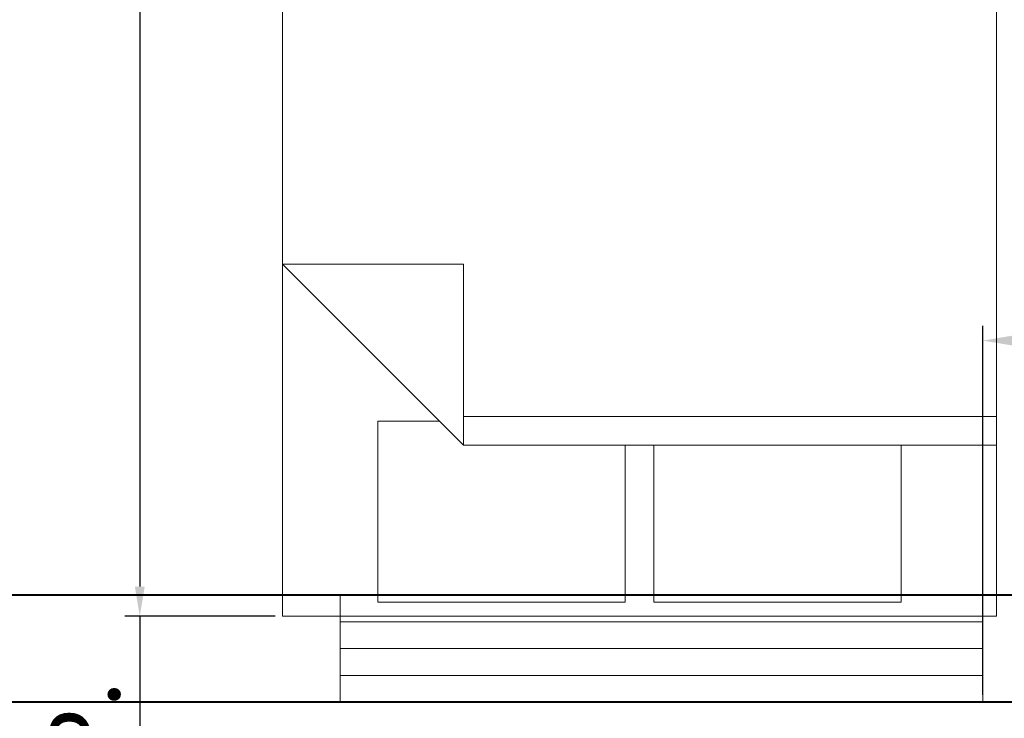
# Model space of a CAD drawing. Units: inches. Extents: x 459864 to 460310, y 324185 to 324787.
# Tile 70 of 112: x 460127 to 460210, y 324282 to 324341. Entities that reach past the tile are written whole.
import ezdxf

# ---------------------------------------------------------------- set-up
doc = ezdxf.new("R2010")
doc.units = ezdxf.units.IN
for name, color, linetype, lineweight in [('A-ANNO-DIMS', 2, 'Continuous', 18), ('A-FURN', 8, 'Continuous', 18), ('A-GLAZ', 4, 'Continuous', 18), ('A-WALL', 7, 'Continuous', 40), ('L-SITE-PATT', 252, 'Continuous', 13)]:
    doc.layers.add(name, color=color, linetype=linetype, lineweight=lineweight)
doc.styles.get("Standard").update_dxf_attribs({"font": 'arial.ttf'})
doc.dimstyles.new('ISO-25', dxfattribs={"dimtxt": 6, "dimasz": 2.5, "dimexe": 1.25, "dimexo": 0.625, "dimtad": 1, "dimdec": 1, "dimlunit": 3, "dimtxsty": 'Standard', "dimcen": 2.5, "dimadec": 0, "dimazin": 0, "dimtfac": 1, "dimtdec": 1, "dimtmove": 0, "dimatfit": 3, "dimfxl": 1, "dimarcsym": 0})

# ---------------------------------------------------------------- blocks, each defined once
blk = doc.blocks.new('Window - Wood Frame 36 in. Wide plan')
for p, q in [((0, 6), (0, 0)), ((36, 6), (36, 0)), ((0, 4.5), (36, 4.5)), ((0, 3), (36, 3)), ((0, 1.5), (36, 1.5))]:
    blk.add_line(p, q)
blk = doc.blocks.new('Bed - Queen')
for p, q in [((0, -80.00003), (0, 0)), ((0, 0), (59.99999, 0)), ((59.99999, 0), (59.99999, -80.00003)), ((7.99999, -1.2), (28.79998, -1.2)), ((7.99999, -14.4), (7.99999, -1.2)), ((28.79998, -1.2), (28.79998, -14.4)), ((31.19999, -1.2), (51.99999, -1.2)), ((31.19999, -14.4), (31.19999, -1.2)), ((51.99999, -1.2), (51.99999, -16.4)), ((0, -14.4), (44.8, -14.4)), ((59.99999, -29.6), (44.8, -14.4)), ((44.8, -14.4), (44.8, -29.6)), ((51.99999, -16.4), (46.79936, -16.4)), ((44.8, -16.8), (0, -16.8)), ((44.8, -29.6), (59.99999, -29.6)), ((59.99999, -80.00003), (0, -80.00003))]:
    blk.add_line(p, q)
blk = doc.blocks.new('*D28')
at = {"layer": 'A-ANNO-DIMS', "color": 0, "lineweight": -2, "transparency": 16777216}
for p, q in [((460148.65, 324370.7), (460136.025, 324370.7)), ((460137.275, 324368.2), (460137.275, 324293.2)), ((460148.65, 324290.7), (460136.025, 324290.7)), ((460137.275, 324290.7), (460137.275, 324198.69))]:
    blk.add_line(p, q, dxfattribs=at)
at = {"layer": 'A-ANNO-DIMS', "color": 0, "transparency": 16777216}
for points in [[(460136.858, 324368.2), (460137.692, 324368.2), (460137.275, 324370.7)], [(460136.858, 324293.2), (460137.692, 324293.2), (460137.275, 324290.7)]]:
    blk.add_solid(points, dxfattribs=at)
at = {"layer": 'Defpoints', "color": 0, "transparency": 16777216}
for p in [(460149.275, 324370.7), (460137.275, 324290.7), (460149.275, 324290.7)]:
    blk.add_point(p, dxfattribs=at)
at = {"layer": 'A-ANNO-DIMS', "color": 0, "transparency": 16777216, "insert": (460133.363, 324243.445), "char_height": 6, "attachment_point": 5, "rotation": 90}
blk.add_mtext('QUEEN BED 6\'-8" TYP.', dxfattribs=at)
blk = doc.blocks.new('*D67')
at = {"layer": 'A-ANNO-DIMS', "color": 0, "lineweight": -2, "transparency": 16777216}
for p, q in [((460208.115, 324284.108), (460208.115, 324315.133)), ((460247.115, 324284.108), (460247.115, 324315.133)), ((460210.615, 324313.883), (460244.615, 324313.883))]:
    blk.add_line(p, q, dxfattribs=at)
at = {"layer": 'A-ANNO-DIMS', "color": 0, "transparency": 16777216}
for points in [[(460210.615, 324314.3), (460210.615, 324313.467), (460208.115, 324313.883)], [(460244.615, 324314.3), (460244.615, 324313.467), (460247.115, 324313.883)]]:
    blk.add_solid(points, dxfattribs=at)
at = {"layer": 'Defpoints', "color": 0, "transparency": 16777216}
for p in [(460247.115, 324313.883), (460208.115, 324283.483), (460247.115, 324283.483)]:
    blk.add_point(p, dxfattribs=at)
at = {"layer": 'A-ANNO-DIMS', "color": 0, "transparency": 16777216, "insert": (460227.615, 324317.574), "char_height": 6, "attachment_point": 5}
blk.add_mtext('3\'-3"', dxfattribs=at)

msp = doc.modelspace()

# ---------------------------------------------------------------- hatches: boundary and pattern name
at = {"layer": 'L-SITE-PATT'}
h = msp.add_hatch(dxfattribs=at)
h.set_pattern_fill('DOTS', color=256)
h.paths.add_polyline_path([(460269.804, 324283.483), (460247.115, 324283.483), (460121.929, 324283.483), (460121.929, 324252.473), (460117.429, 324252.473), (460110.124, 324252.473), (460110.124, 324243.287), (460080.83, 324243.287), (460080.83, 324252.473), (460061.115, 324252.473), (460061.115, 324251.882), (460077.909, 324251.882), (460077.909, 324199.483), (460080.83, 324199.483), (460080.83, 324207.553), (460110.124, 324207.553), (460110.124, 324199.483), (460110.813, 324199.483), (460262.115, 324199.483), (460269.804, 324199.483)], flags=17)
edge = h.paths.add_edge_path(flags=0)
edge.add_ellipse((460222.59, 324263.813), major_axis=(-8.485, 8.485), ratio=1, start_angle=405, end_angle=495, ccw=False)
edge.add_line((460214.821, 324254.66), (460214.832, 324254.666))
edge.add_ellipse((460222.59, 324263.813), major_axis=(-8.485, 8.485), ratio=1, start_angle=405, end_angle=495, ccw=False)
edge.add_line((460210.759, 324261.781), (460210.768, 324261.787))
edge.add_ellipse((460222.59, 324263.813), major_axis=(-8.485, 8.485), ratio=1, start_angle=405, end_angle=495, ccw=False)
edge.add_ellipse((460222.59, 324263.813), major_axis=(-8.485, 8.485), ratio=1, start_angle=392.75402, end_angle=405, ccw=False)
edge.add_ellipse((460222.59, 324263.813), major_axis=(-8.485, 8.485), ratio=1, start_angle=380.93472, end_angle=392.75402, ccw=False)
edge.add_line((460211.337, 324267.985), (460211.34, 324267.985))
edge.add_ellipse((460222.59, 324263.813), major_axis=(-8.485, 8.485), ratio=1, start_angle=380.93472, end_angle=392.75402, ccw=False)
edge.add_ellipse((460222.59, 324263.813), major_axis=(-8.485, 8.485), ratio=1, start_angle=347.90152, end_angle=380.93472, ccw=False)
edge.add_ellipse((460222.59, 324263.813), major_axis=(-8.485, 8.485), ratio=1, start_angle=327.06192, end_angle=347.90152, ccw=False)
edge.add_ellipse((460222.59, 324263.813), major_axis=(-8.485, 8.485), ratio=1, start_angle=278.32464, end_angle=327.06192, ccw=False)
edge.add_line((460225.158, 324275.536), (460225.158, 324275.535))
edge.add_ellipse((460222.59, 324263.813), major_axis=(-8.485, 8.485), ratio=1, start_angle=278.32464, end_angle=327.06192, ccw=False)
edge.add_ellipse((460222.59, 324263.813), major_axis=(-8.485, 8.485), ratio=1, start_angle=260.64357, end_angle=278.32464, ccw=False)
edge.add_ellipse((460222.59, 324263.813), major_axis=(-8.485, 8.485), ratio=1, start_angle=225, end_angle=260.64357, ccw=False)
edge.add_line((460234.509, 324265.243), (460234.501, 324265.239))
edge.add_ellipse((460222.59, 324263.813), major_axis=(-8.485, 8.485), ratio=1, start_angle=225, end_angle=260.64357, ccw=False)
edge.add_ellipse((460222.59, 324263.813), major_axis=(-8.485, 8.485), ratio=1, start_angle=495, end_angle=585, ccw=False)
edge.add_line((460234.437, 324261.861), (460234.424, 324261.858))
edge.add_ellipse((460222.59, 324263.813), major_axis=(-8.485, 8.485), ratio=1, start_angle=495, end_angle=585, ccw=False)
edge.add_line((460227.95, 324253.067), (460227.946, 324253.083))
edge.add_ellipse((460222.59, 324263.813), major_axis=(-8.485, 8.485), ratio=1, start_angle=495, end_angle=585, ccw=False)
edge.add_line((460226.223, 324252.369), (460226.211, 324252.38))
edge.add_ellipse((460222.59, 324263.813), major_axis=(-8.485, 8.485), ratio=1, start_angle=495, end_angle=585, ccw=False)
h.paths.add_polyline_path([(460219.651, 324254.347), (460218.461, 324253.545), (460218.275, 324254.789), (460219.642, 324256.542), (460219.625, 324260.848), (460216.11, 324257.333), (460214.35, 324256.978), (460215.416, 324259.356), (460212.524, 324258.496), (460213.137, 324259.93), (460218.507, 324263.813), (460222.59, 324263.813), (460222.59, 324267.807), (460218.176, 324272.212), (460219.026, 324274.639), (460222.59, 324272.811), (460222.59, 324275.423), (460223.057, 324274.825), (460222.675, 324273.492), (460225.912, 324267.135), (460219.625, 324260.848)], flags=0)
edge = h.paths.add_edge_path(flags=0)
edge.add_ellipse((460194.576, 324264.046), major_axis=(-8.485, 8.485), ratio=1, start_angle=495, end_angle=585, ccw=False)
edge.add_line((460199.936, 324253.3), (460199.932, 324253.316))
edge.add_ellipse((460194.576, 324264.046), major_axis=(-8.485, 8.485), ratio=1, start_angle=495, end_angle=585, ccw=False)
edge.add_line((460198.208, 324252.603), (460198.196, 324252.613))
edge.add_ellipse((460194.576, 324264.046), major_axis=(-8.485, 8.485), ratio=1, start_angle=495, end_angle=585, ccw=False)
edge.add_ellipse((460194.576, 324264.046), major_axis=(-8.485, 8.485), ratio=1, start_angle=405, end_angle=495, ccw=False)
edge.add_line((460186.806, 324254.893), (460186.817, 324254.899))
edge.add_ellipse((460194.576, 324264.046), major_axis=(-8.485, 8.485), ratio=1, start_angle=405, end_angle=495, ccw=False)
edge.add_line((460182.744, 324262.014), (460182.753, 324262.02))
edge.add_ellipse((460194.576, 324264.046), major_axis=(-8.485, 8.485), ratio=1, start_angle=405, end_angle=495, ccw=False)
edge.add_ellipse((460194.576, 324264.046), major_axis=(-8.485, 8.485), ratio=1, start_angle=392.75402, end_angle=405, ccw=False)
edge.add_ellipse((460194.576, 324264.046), major_axis=(-8.485, 8.485), ratio=1, start_angle=380.93472, end_angle=392.75402, ccw=False)
edge.add_line((460183.323, 324268.218), (460183.326, 324268.218))
edge.add_ellipse((460194.576, 324264.046), major_axis=(-8.485, 8.485), ratio=1, start_angle=380.93472, end_angle=392.75402, ccw=False)
edge.add_ellipse((460194.576, 324264.046), major_axis=(-8.485, 8.485), ratio=1, start_angle=347.90152, end_angle=380.93472, ccw=False)
edge.add_ellipse((460194.576, 324264.046), major_axis=(-8.485, 8.485), ratio=1, start_angle=327.06192, end_angle=347.90152, ccw=False)
edge.add_ellipse((460194.576, 324264.046), major_axis=(-8.485, 8.485), ratio=1, start_angle=278.32464, end_angle=327.06192, ccw=False)
edge.add_line((460197.144, 324275.769), (460197.143, 324275.768))
edge.add_ellipse((460194.576, 324264.046), major_axis=(-8.485, 8.485), ratio=1, start_angle=278.32464, end_angle=327.06192, ccw=False)
edge.add_ellipse((460194.576, 324264.046), major_axis=(-8.485, 8.485), ratio=1, start_angle=260.64357, end_angle=278.32464, ccw=False)
edge.add_ellipse((460194.576, 324264.046), major_axis=(-8.485, 8.485), ratio=1, start_angle=225, end_angle=260.64357, ccw=False)
edge.add_line((460206.494, 324265.476), (460206.487, 324265.473))
edge.add_ellipse((460194.576, 324264.046), major_axis=(-8.485, 8.485), ratio=1, start_angle=225, end_angle=260.64357, ccw=False)
edge.add_ellipse((460194.576, 324264.046), major_axis=(-8.485, 8.485), ratio=1, start_angle=495, end_angle=585, ccw=False)
edge.add_line((460206.422, 324262.094), (460206.409, 324262.091))
h.paths.add_polyline_path([(460191.61, 324261.081), (460191.637, 324254.58), (460190.447, 324253.778), (460190.261, 324255.023), (460191.628, 324256.775), (460191.61, 324261.081), (460188.096, 324257.566), (460186.335, 324257.211), (460187.402, 324259.589), (460184.509, 324258.729), (460185.123, 324260.163), (460190.493, 324264.046), (460194.576, 324264.046), (460194.576, 324268.04), (460190.161, 324272.446), (460191.011, 324274.872), (460194.576, 324273.044), (460194.576, 324275.657), (460195.043, 324275.058), (460194.661, 324273.725), (460197.897, 324267.368)], flags=0)
edge = h.paths.add_edge_path(flags=0)
edge.add_ellipse((460252.912, 324263.578), major_axis=(-8.485, 8.485), ratio=1, start_angle=405, end_angle=495, ccw=False)
edge.add_line((460241.081, 324261.545), (460241.089, 324261.551))
edge.add_ellipse((460252.912, 324263.578), major_axis=(-8.485, 8.485), ratio=1, start_angle=405, end_angle=495, ccw=False)
edge.add_ellipse((460252.912, 324263.578), major_axis=(-8.485, 8.485), ratio=1, start_angle=392.75402, end_angle=405, ccw=False)
edge.add_ellipse((460252.912, 324263.578), major_axis=(-8.485, 8.485), ratio=1, start_angle=380.93472, end_angle=392.75402, ccw=False)
edge.add_line((460241.659, 324267.749), (460241.662, 324267.749))
edge.add_ellipse((460252.912, 324263.578), major_axis=(-8.485, 8.485), ratio=1, start_angle=380.93472, end_angle=392.75402, ccw=False)
edge.add_ellipse((460252.912, 324263.578), major_axis=(-8.485, 8.485), ratio=1, start_angle=347.90152, end_angle=380.93472, ccw=False)
edge.add_ellipse((460252.912, 324263.578), major_axis=(-8.485, 8.485), ratio=1, start_angle=327.06192, end_angle=347.90152, ccw=False)
edge.add_ellipse((460252.912, 324263.578), major_axis=(-8.485, 8.485), ratio=1, start_angle=278.32464, end_angle=327.06192, ccw=False)
edge.add_line((460255.48, 324275.3), (460255.479, 324275.299))
edge.add_ellipse((460252.912, 324263.578), major_axis=(-8.485, 8.485), ratio=1, start_angle=278.32464, end_angle=327.06192, ccw=False)
edge.add_ellipse((460252.912, 324263.578), major_axis=(-8.485, 8.485), ratio=1, start_angle=260.64357, end_angle=278.32464, ccw=False)
edge.add_ellipse((460252.912, 324263.578), major_axis=(-8.485, 8.485), ratio=1, start_angle=225, end_angle=260.64357, ccw=False)
edge.add_line((460264.83, 324265.007), (460264.823, 324265.004))
edge.add_ellipse((460252.912, 324263.578), major_axis=(-8.485, 8.485), ratio=1, start_angle=225, end_angle=260.64357, ccw=False)
edge.add_ellipse((460252.912, 324263.578), major_axis=(-8.485, 8.485), ratio=1, start_angle=495, end_angle=585, ccw=False)
edge.add_line((460264.758, 324261.626), (460264.745, 324261.622))
edge.add_ellipse((460252.912, 324263.578), major_axis=(-8.485, 8.485), ratio=1, start_angle=495, end_angle=585, ccw=False)
edge.add_line((460258.272, 324252.832), (460258.268, 324252.848))
edge.add_ellipse((460252.912, 324263.578), major_axis=(-8.485, 8.485), ratio=1, start_angle=495, end_angle=585, ccw=False)
edge.add_line((460256.545, 324252.134), (460256.533, 324252.144))
edge.add_ellipse((460252.912, 324263.578), major_axis=(-8.485, 8.485), ratio=1, start_angle=495, end_angle=585, ccw=False)
edge.add_ellipse((460252.912, 324263.578), major_axis=(-8.485, 8.485), ratio=1, start_angle=405, end_angle=495, ccw=False)
edge.add_line((460245.143, 324254.424), (460245.153, 324254.43))
h.paths.add_polyline_path([(460244.672, 324256.742), (460245.738, 324259.12), (460242.846, 324258.26), (460243.459, 324259.694), (460248.829, 324263.578), (460252.912, 324263.578), (460252.912, 324267.571), (460248.497, 324271.977), (460249.348, 324274.403), (460252.912, 324272.576), (460252.912, 324275.188), (460253.379, 324274.589), (460252.997, 324273.257), (460256.233, 324266.899), (460249.946, 324260.612), (460249.973, 324254.111), (460248.783, 324253.309), (460248.597, 324254.554), (460249.964, 324256.306), (460249.946, 324260.612), (460246.432, 324257.097)], flags=0)
edge = h.paths.add_edge_path(flags=0)
edge.add_ellipse((460167.439, 324262.833), major_axis=(-8.485, 8.485), ratio=1, start_angle=495, end_angle=585, ccw=False)
edge.add_line((460172.799, 324252.087), (460172.795, 324252.103))
edge.add_ellipse((460167.439, 324262.833), major_axis=(-8.485, 8.485), ratio=1, start_angle=495, end_angle=585, ccw=False)
edge.add_line((460171.071, 324251.389), (460171.059, 324251.399))
edge.add_ellipse((460167.439, 324262.833), major_axis=(-8.485, 8.485), ratio=1, start_angle=495, end_angle=585, ccw=False)
edge.add_ellipse((460167.439, 324262.833), major_axis=(-8.485, 8.485), ratio=1, start_angle=405, end_angle=495, ccw=False)
edge.add_line((460159.669, 324253.679), (460159.68, 324253.685))
edge.add_ellipse((460167.439, 324262.833), major_axis=(-8.485, 8.485), ratio=1, start_angle=405, end_angle=495, ccw=False)
edge.add_line((460155.607, 324260.8), (460155.616, 324260.806))
edge.add_ellipse((460167.439, 324262.833), major_axis=(-8.485, 8.485), ratio=1, start_angle=405, end_angle=495, ccw=False)
edge.add_ellipse((460167.439, 324262.833), major_axis=(-8.485, 8.485), ratio=1, start_angle=392.75402, end_angle=405, ccw=False)
edge.add_ellipse((460167.439, 324262.833), major_axis=(-8.485, 8.485), ratio=1, start_angle=380.93472, end_angle=392.75402, ccw=False)
edge.add_line((460156.185, 324267.005), (460156.189, 324267.005))
edge.add_ellipse((460167.439, 324262.833), major_axis=(-8.485, 8.485), ratio=1, start_angle=380.93472, end_angle=392.75402, ccw=False)
edge.add_ellipse((460167.439, 324262.833), major_axis=(-8.485, 8.485), ratio=1, start_angle=347.90152, end_angle=380.93472, ccw=False)
edge.add_ellipse((460167.439, 324262.833), major_axis=(-8.485, 8.485), ratio=1, start_angle=327.06192, end_angle=347.90152, ccw=False)
edge.add_ellipse((460167.439, 324262.833), major_axis=(-8.485, 8.485), ratio=1, start_angle=278.32464, end_angle=327.06192, ccw=False)
edge.add_line((460170.007, 324274.556), (460170.006, 324274.554))
edge.add_ellipse((460167.439, 324262.833), major_axis=(-8.485, 8.485), ratio=1, start_angle=278.32464, end_angle=327.06192, ccw=False)
edge.add_ellipse((460167.439, 324262.833), major_axis=(-8.485, 8.485), ratio=1, start_angle=260.64357, end_angle=278.32464, ccw=False)
edge.add_ellipse((460167.439, 324262.833), major_axis=(-8.485, 8.485), ratio=1, start_angle=225, end_angle=260.64357, ccw=False)
edge.add_line((460179.357, 324264.262), (460179.35, 324264.259))
edge.add_ellipse((460167.439, 324262.833), major_axis=(-8.485, 8.485), ratio=1, start_angle=225, end_angle=260.64357, ccw=False)
edge.add_ellipse((460167.439, 324262.833), major_axis=(-8.485, 8.485), ratio=1, start_angle=495, end_angle=585, ccw=False)
edge.add_line((460179.285, 324260.881), (460179.272, 324260.877))
h.paths.add_polyline_path([(460164.473, 324259.867), (460164.5, 324253.366), (460163.31, 324252.565), (460163.124, 324253.809), (460164.491, 324255.561), (460164.473, 324259.867), (460160.958, 324256.353), (460159.198, 324255.998), (460160.265, 324258.375), (460157.372, 324257.515), (460157.986, 324258.949), (460163.356, 324262.833), (460167.439, 324262.833), (460167.439, 324266.826), (460163.024, 324271.232), (460163.874, 324273.659), (460167.439, 324271.831), (460167.439, 324274.443), (460167.905, 324273.844), (460167.524, 324272.512), (460170.76, 324266.154)], flags=0)
edge = h.paths.add_edge_path(flags=0)
edge.add_ellipse((460140.758, 324262.37), major_axis=(-8.485, 8.485), ratio=1, start_angle=495, end_angle=585, ccw=False)
edge.add_line((460146.118, 324251.624), (460146.114, 324251.639))
edge.add_ellipse((460140.758, 324262.37), major_axis=(-8.485, 8.485), ratio=1, start_angle=495, end_angle=585, ccw=False)
edge.add_line((460144.391, 324250.926), (460144.379, 324250.936))
edge.add_ellipse((460140.758, 324262.37), major_axis=(-8.485, 8.485), ratio=1, start_angle=495, end_angle=585, ccw=False)
edge.add_ellipse((460140.758, 324262.37), major_axis=(-8.485, 8.485), ratio=1, start_angle=405, end_angle=495, ccw=False)
edge.add_line((460132.989, 324253.216), (460132.999, 324253.222))
edge.add_ellipse((460140.758, 324262.37), major_axis=(-8.485, 8.485), ratio=1, start_angle=405, end_angle=495, ccw=False)
edge.add_line((460128.927, 324260.337), (460128.935, 324260.343))
edge.add_ellipse((460140.758, 324262.37), major_axis=(-8.485, 8.485), ratio=1, start_angle=405, end_angle=495, ccw=False)
edge.add_ellipse((460140.758, 324262.37), major_axis=(-8.485, 8.485), ratio=1, start_angle=392.75402, end_angle=405, ccw=False)
edge.add_ellipse((460140.758, 324262.37), major_axis=(-8.485, 8.485), ratio=1, start_angle=380.93472, end_angle=392.75402, ccw=False)
edge.add_line((460129.505, 324266.541), (460129.508, 324266.541))
edge.add_ellipse((460140.758, 324262.37), major_axis=(-8.485, 8.485), ratio=1, start_angle=380.93472, end_angle=392.75402, ccw=False)
edge.add_ellipse((460140.758, 324262.37), major_axis=(-8.485, 8.485), ratio=1, start_angle=347.90152, end_angle=380.93472, ccw=False)
edge.add_ellipse((460140.758, 324262.37), major_axis=(-8.485, 8.485), ratio=1, start_angle=327.06192, end_angle=347.90152, ccw=False)
edge.add_ellipse((460140.758, 324262.37), major_axis=(-8.485, 8.485), ratio=1, start_angle=278.32464, end_angle=327.06192, ccw=False)
edge.add_line((460143.326, 324274.092), (460143.325, 324274.091))
edge.add_ellipse((460140.758, 324262.37), major_axis=(-8.485, 8.485), ratio=1, start_angle=278.32464, end_angle=327.06192, ccw=False)
edge.add_ellipse((460140.758, 324262.37), major_axis=(-8.485, 8.485), ratio=1, start_angle=260.64357, end_angle=278.32464, ccw=False)
edge.add_ellipse((460140.758, 324262.37), major_axis=(-8.485, 8.485), ratio=1, start_angle=225, end_angle=260.64357, ccw=False)
edge.add_line((460152.677, 324263.799), (460152.669, 324263.796))
edge.add_ellipse((460140.758, 324262.37), major_axis=(-8.485, 8.485), ratio=1, start_angle=225, end_angle=260.64357, ccw=False)
edge.add_ellipse((460140.758, 324262.37), major_axis=(-8.485, 8.485), ratio=1, start_angle=495, end_angle=585, ccw=False)
edge.add_line((460152.604, 324260.418), (460152.592, 324260.414))
h.paths.add_polyline_path([(460137.792, 324259.404), (460137.819, 324252.903), (460136.629, 324252.101), (460136.443, 324253.346), (460137.81, 324255.098), (460137.792, 324259.404), (460134.278, 324255.889), (460132.518, 324255.534), (460133.584, 324257.912), (460130.692, 324257.052), (460131.305, 324258.486), (460136.675, 324262.37), (460140.758, 324262.37), (460140.758, 324266.363), (460136.343, 324270.769), (460137.194, 324273.195), (460140.758, 324271.367), (460140.758, 324273.98), (460141.225, 324273.381), (460140.843, 324272.049), (460144.079, 324265.691)], flags=0)
h.paths.add_polyline_path([(460110.124, 324227.414), (460080.83, 324227.414), (460080.83, 324235.484), (460110.124, 324235.484)], flags=16)
h.paths.add_polyline_path([(460110.124, 324220.797), (460110.124, 324212.727), (460080.83, 324212.727), (460080.83, 324220.797)], flags=16)
h.paths.add_polyline_path([(460269.804, 324283.483), (460247.115, 324283.483), (460121.929, 324283.483), (460121.929, 324252.473), (460117.429, 324252.473), (460110.124, 324252.473), (460110.124, 324243.287), (460080.83, 324243.287), (460080.83, 324252.473), (460061.115, 324252.473), (460061.115, 324251.882), (460077.909, 324251.882), (460077.909, 324199.483), (460080.83, 324199.483), (460080.83, 324207.553), (460110.124, 324207.553), (460110.124, 324199.483), (460262.115, 324199.483), (460269.804, 324199.483)], flags=17)
h.paths.add_polyline_path([(460219.651, 324254.347), (460218.461, 324253.545), (460218.275, 324254.789), (460219.642, 324256.542), (460219.625, 324260.848), (460216.11, 324257.333), (460214.35, 324256.978), (460215.416, 324259.356), (460212.524, 324258.496), (460213.137, 324259.93), (460218.507, 324263.813), (460222.59, 324263.813), (460220.18, 324266.223), (460215.461, 324265.308), (460211.835, 324266.137), (460216.247, 324267.985), (460218.418, 324267.985), (460222.59, 324263.813), (460222.59, 324267.807), (460218.176, 324272.212), (460219.026, 324274.639), (460222.59, 324272.811), (460222.59, 324275.423), (460223.057, 324274.825), (460222.675, 324273.492), (460225.912, 324267.135), (460222.59, 324263.813), (460231.383, 324263.813), (460228.485, 324262.488), (460224.425, 324261.978), (460228.68, 324257.724), (460228.966, 324254.791), (460227.142, 324256.537), (460227.542, 324254.819), (460227.333, 324253.614), (460222.59, 324259.985), (460222.59, 324255.497), (460221.377, 324256.541), (460220.576, 324261.799), (460219.625, 324260.848)], flags=0)
h.paths.add_polyline_path([(460199.127, 324256.77), (460199.528, 324255.052), (460199.319, 324253.848), (460194.576, 324260.218), (460194.576, 324255.73), (460193.363, 324256.774), (460192.561, 324262.032), (460191.61, 324261.081), (460191.637, 324254.58), (460190.447, 324253.778), (460190.261, 324255.023), (460191.628, 324256.775), (460191.61, 324261.081), (460188.096, 324257.566), (460186.335, 324257.211), (460187.402, 324259.589), (460184.509, 324258.729), (460185.123, 324260.163), (460190.493, 324264.046), (460194.576, 324264.046), (460192.166, 324266.456), (460187.446, 324265.541), (460183.82, 324266.37), (460188.232, 324268.218), (460190.404, 324268.218), (460194.576, 324264.046), (460194.576, 324268.04), (460190.161, 324272.446), (460191.011, 324274.872), (460194.576, 324273.044), (460194.576, 324275.657), (460195.043, 324275.058), (460194.661, 324273.725), (460197.897, 324267.368), (460194.576, 324264.046), (460203.368, 324264.046), (460200.47, 324262.721), (460196.411, 324262.212), (460200.665, 324257.957), (460200.951, 324255.024)], flags=0)
h.paths.add_polyline_path([(460244.672, 324256.742), (460245.738, 324259.12), (460242.846, 324258.26), (460243.459, 324259.694), (460248.829, 324263.578), (460252.912, 324263.578), (460250.502, 324265.987), (460245.783, 324265.072), (460242.156, 324265.901), (460246.568, 324267.749), (460248.74, 324267.749), (460252.912, 324263.578), (460252.912, 324267.571), (460248.497, 324271.977), (460249.348, 324274.403), (460252.912, 324272.576), (460252.912, 324275.188), (460253.379, 324274.589), (460252.997, 324273.257), (460256.233, 324266.899), (460252.912, 324263.578), (460261.705, 324263.578), (460258.806, 324262.252), (460254.747, 324261.743), (460259.002, 324257.488), (460259.288, 324254.555), (460257.463, 324256.301), (460257.864, 324254.583), (460257.655, 324253.379), (460252.912, 324259.749), (460252.912, 324255.261), (460251.699, 324256.305), (460250.897, 324261.563), (460249.946, 324260.612), (460249.973, 324254.111), (460248.783, 324253.309), (460248.597, 324254.554), (460249.964, 324256.306), (460249.946, 324260.612), (460246.432, 324257.097)], flags=0)
h.paths.add_polyline_path([(460173.528, 324256.743), (460173.814, 324253.811), (460171.99, 324255.556), (460172.39, 324253.838), (460172.182, 324252.634), (460167.439, 324259.004), (460167.439, 324254.516), (460166.226, 324255.56), (460165.424, 324260.818), (460164.473, 324259.867), (460164.5, 324253.366), (460163.31, 324252.565), (460163.124, 324253.809), (460164.491, 324255.561), (460164.473, 324259.867), (460160.958, 324256.353), (460159.198, 324255.998), (460160.265, 324258.375), (460157.372, 324257.515), (460157.986, 324258.949), (460163.356, 324262.833), (460167.439, 324262.833), (460165.029, 324265.243), (460160.309, 324264.327), (460156.683, 324265.156), (460161.095, 324267.005), (460163.267, 324267.005), (460167.439, 324262.833), (460167.439, 324266.826), (460163.024, 324271.232), (460163.874, 324273.659), (460167.439, 324271.831), (460167.439, 324274.443), (460167.905, 324273.844), (460167.524, 324272.512), (460170.76, 324266.154), (460167.439, 324262.833), (460176.231, 324262.833), (460173.333, 324261.507), (460169.274, 324260.998)], flags=0)
h.paths.add_polyline_path([(460146.848, 324256.28), (460147.134, 324253.347), (460145.31, 324255.093), (460145.71, 324253.375), (460145.501, 324252.171), (460140.758, 324258.541), (460140.758, 324254.053), (460139.545, 324255.097), (460138.744, 324260.355), (460137.792, 324259.404), (460137.819, 324252.903), (460136.629, 324252.101), (460136.443, 324253.346), (460137.81, 324255.098), (460137.792, 324259.404), (460134.278, 324255.889), (460132.518, 324255.534), (460133.584, 324257.912), (460130.692, 324257.052), (460131.305, 324258.486), (460136.675, 324262.37), (460140.758, 324262.37), (460138.348, 324264.779), (460133.629, 324263.864), (460130.002, 324264.693), (460134.414, 324266.541), (460136.586, 324266.541), (460140.758, 324262.37), (460140.758, 324266.363), (460136.343, 324270.769), (460137.194, 324273.195), (460140.758, 324271.367), (460140.758, 324273.98), (460141.225, 324273.381), (460140.843, 324272.049), (460144.079, 324265.691), (460140.758, 324262.37), (460149.551, 324262.37), (460146.653, 324261.044), (460142.593, 324260.535)], flags=0)
edge = h.paths.add_edge_path()
edge.add_line((460269.804, 324272.549), (460260.881, 324272.549))
edge.add_ellipse((460252.912, 324263.578), major_axis=(-8.485, 8.485), ratio=1, start_angle=260.64357, end_angle=273.38462, ccw=False)
edge.add_line((460262.283, 324271.092), (460262.261, 324271.091))
edge.add_ellipse((460252.912, 324263.578), major_axis=(-8.485, 8.485), ratio=1, start_angle=260.64357, end_angle=273.38462, ccw=False)
edge.add_ellipse((460252.912, 324263.578), major_axis=(-8.485, 8.485), ratio=1, start_angle=225, end_angle=260.64357, ccw=False)
edge.add_line((460263.609, 324269.063), (460263.572, 324269.058))
edge.add_ellipse((460252.912, 324263.578), major_axis=(-8.485, 8.485), ratio=1, start_angle=225, end_angle=260.64357, ccw=False)
edge.add_line((460264.615, 324266.306), (460264.585, 324266.305))
edge.add_ellipse((460252.912, 324263.578), major_axis=(-8.485, 8.485), ratio=1, start_angle=225, end_angle=260.64357, ccw=False)
edge.add_line((460264.83, 324265.007), (460264.823, 324265.004))
edge.add_ellipse((460252.912, 324263.578), major_axis=(-8.485, 8.485), ratio=1, start_angle=225, end_angle=260.64357, ccw=False)
edge.add_ellipse((460252.912, 324263.578), major_axis=(-8.485, 8.485), ratio=1, start_angle=495, end_angle=585, ccw=False)
edge.add_line((460264.758, 324261.626), (460264.745, 324261.622))
edge.add_ellipse((460252.912, 324263.578), major_axis=(-8.485, 8.485), ratio=1, start_angle=495, end_angle=585, ccw=False)
edge.add_line((460263.442, 324257.739), (460263.389, 324257.779))
edge.add_ellipse((460252.912, 324263.578), major_axis=(-8.485, 8.485), ratio=1, start_angle=495, end_angle=585, ccw=False)
edge.add_line((460258.128, 324252.744), (460258.102, 324252.779))
edge.add_ellipse((460252.912, 324263.578), major_axis=(-8.485, 8.485), ratio=1, start_angle=495, end_angle=585, ccw=False)
edge.add_line((460256.545, 324252.134), (460256.533, 324252.144))
edge.add_ellipse((460252.912, 324263.578), major_axis=(-8.485, 8.485), ratio=1, start_angle=495, end_angle=585, ccw=False)
edge.add_ellipse((460252.912, 324263.578), major_axis=(-8.485, 8.485), ratio=1, start_angle=405, end_angle=495, ccw=False)
edge.add_line((460250.594, 324251.78), (460250.605, 324251.82))
edge.add_ellipse((460252.912, 324263.578), major_axis=(-8.485, 8.485), ratio=1, start_angle=405, end_angle=495, ccw=False)
edge.add_line((460245.143, 324254.424), (460245.153, 324254.43))
edge.add_ellipse((460252.912, 324263.578), major_axis=(-8.485, 8.485), ratio=1, start_angle=405, end_angle=495, ccw=False)
edge.add_line((460243.525, 324256.059), (460243.56, 324256.091))
edge.add_ellipse((460252.912, 324263.578), major_axis=(-8.485, 8.485), ratio=1, start_angle=405, end_angle=495, ccw=False)
edge.add_line((460241.44, 324259.893), (460241.522, 324259.896))
edge.add_ellipse((460252.912, 324263.578), major_axis=(-8.485, 8.485), ratio=1, start_angle=405, end_angle=495, ccw=False)
edge.add_line((460241.081, 324261.545), (460241.089, 324261.551))
edge.add_ellipse((460252.912, 324263.578), major_axis=(-8.485, 8.485), ratio=1, start_angle=405, end_angle=495, ccw=False)
edge.add_ellipse((460252.912, 324263.578), major_axis=(-8.485, 8.485), ratio=1, start_angle=392.75402, end_angle=405, ccw=False)
edge.add_line((460241.05, 324265.438), (460241.063, 324265.443))
edge.add_ellipse((460252.912, 324263.578), major_axis=(-8.485, 8.485), ratio=1, start_angle=392.75402, end_angle=405, ccw=False)
edge.add_ellipse((460252.912, 324263.578), major_axis=(-8.485, 8.485), ratio=1, start_angle=380.93472, end_angle=392.75402, ccw=False)
edge.add_line((460241.452, 324267.176), (460241.469, 324267.171))
edge.add_ellipse((460252.912, 324263.578), major_axis=(-8.485, 8.485), ratio=1, start_angle=380.93472, end_angle=392.75402, ccw=False)
edge.add_line((460241.659, 324267.749), (460241.662, 324267.749))
edge.add_ellipse((460252.912, 324263.578), major_axis=(-8.485, 8.485), ratio=1, start_angle=380.93472, end_angle=392.75402, ccw=False)
edge.add_ellipse((460252.912, 324263.578), major_axis=(-8.485, 8.485), ratio=1, start_angle=356.61538, end_angle=380.93472, ccw=False)
edge.add_line((460244.88, 324272.488), (460244.713, 324272.549))
edge.add_line((460244.713, 324272.549), (460230.817, 324272.549))
edge.add_ellipse((460222.59, 324263.813), major_axis=(-8.485, 8.485), ratio=1, start_angle=260.64357, end_angle=271.71777, ccw=False)
edge.add_ellipse((460222.59, 324263.813), major_axis=(-8.485, 8.485), ratio=1, start_angle=225, end_angle=260.64357, ccw=False)
edge.add_line((460233.287, 324269.299), (460233.25, 324269.294))
edge.add_ellipse((460222.59, 324263.813), major_axis=(-8.485, 8.485), ratio=1, start_angle=225, end_angle=260.64357, ccw=False)
edge.add_line((460234.294, 324266.541), (460234.264, 324266.541))
edge.add_ellipse((460222.59, 324263.813), major_axis=(-8.485, 8.485), ratio=1, start_angle=225, end_angle=260.64357, ccw=False)
edge.add_line((460234.509, 324265.243), (460234.501, 324265.239))
edge.add_ellipse((460222.59, 324263.813), major_axis=(-8.485, 8.485), ratio=1, start_angle=225, end_angle=260.64357, ccw=False)
edge.add_ellipse((460222.59, 324263.813), major_axis=(-8.485, 8.485), ratio=1, start_angle=495, end_angle=585, ccw=False)
edge.add_line((460234.437, 324261.861), (460234.424, 324261.858))
edge.add_ellipse((460222.59, 324263.813), major_axis=(-8.485, 8.485), ratio=1, start_angle=495, end_angle=585, ccw=False)
edge.add_line((460233.121, 324257.975), (460233.068, 324258.015))
edge.add_ellipse((460222.59, 324263.813), major_axis=(-8.485, 8.485), ratio=1, start_angle=495, end_angle=585, ccw=False)
edge.add_line((460227.806, 324252.979), (460227.78, 324253.014))
edge.add_ellipse((460222.59, 324263.813), major_axis=(-8.485, 8.485), ratio=1, start_angle=495, end_angle=585, ccw=False)
edge.add_line((460226.223, 324252.369), (460226.211, 324252.38))
edge.add_ellipse((460222.59, 324263.813), major_axis=(-8.485, 8.485), ratio=1, start_angle=495, end_angle=585, ccw=False)
edge.add_ellipse((460222.59, 324263.813), major_axis=(-8.485, 8.485), ratio=1, start_angle=405, end_angle=495, ccw=False)
edge.add_line((460220.272, 324252.016), (460220.283, 324252.055))
edge.add_ellipse((460222.59, 324263.813), major_axis=(-8.485, 8.485), ratio=1, start_angle=405, end_angle=495, ccw=False)
edge.add_line((460214.821, 324254.66), (460214.832, 324254.666))
edge.add_ellipse((460222.59, 324263.813), major_axis=(-8.485, 8.485), ratio=1, start_angle=405, end_angle=495, ccw=False)
edge.add_line((460213.203, 324256.295), (460213.239, 324256.327))
edge.add_ellipse((460222.59, 324263.813), major_axis=(-8.485, 8.485), ratio=1, start_angle=405, end_angle=495, ccw=False)
edge.add_line((460211.118, 324260.128), (460211.201, 324260.131))
edge.add_ellipse((460222.59, 324263.813), major_axis=(-8.485, 8.485), ratio=1, start_angle=405, end_angle=495, ccw=False)
edge.add_line((460210.759, 324261.781), (460210.768, 324261.787))
edge.add_ellipse((460222.59, 324263.813), major_axis=(-8.485, 8.485), ratio=1, start_angle=405, end_angle=495, ccw=False)
edge.add_ellipse((460222.59, 324263.813), major_axis=(-8.485, 8.485), ratio=1, start_angle=392.75402, end_angle=405, ccw=False)
edge.add_line((460210.729, 324265.673), (460210.741, 324265.678))
edge.add_ellipse((460222.59, 324263.813), major_axis=(-8.485, 8.485), ratio=1, start_angle=392.75402, end_angle=405, ccw=False)
edge.add_ellipse((460222.59, 324263.813), major_axis=(-8.485, 8.485), ratio=1, start_angle=380.93472, end_angle=392.75402, ccw=False)
edge.add_line((460211.13, 324267.412), (460211.147, 324267.407))
edge.add_ellipse((460222.59, 324263.813), major_axis=(-8.485, 8.485), ratio=1, start_angle=380.93472, end_angle=392.75402, ccw=False)
edge.add_line((460211.337, 324267.985), (460211.34, 324267.985))
edge.add_ellipse((460222.59, 324263.813), major_axis=(-8.485, 8.485), ratio=1, start_angle=380.93472, end_angle=392.75402, ccw=False)
edge.add_ellipse((460222.59, 324263.813), major_axis=(-8.485, 8.485), ratio=1, start_angle=358.28223, end_angle=380.93472, ccw=False)
edge.add_line((460213.705, 324271.902), (460213.709, 324271.869))
edge.add_ellipse((460222.59, 324263.813), major_axis=(-8.485, 8.485), ratio=1, start_angle=358.28223, end_angle=380.93472, ccw=False)
edge.add_line((460214.363, 324272.549), (460203.078, 324272.549))
edge.add_line((460203.078, 324272.549), (460203.06, 324272.531))
edge.add_ellipse((460194.576, 324264.046), major_axis=(-8.485, 8.485), ratio=1, start_angle=260.64357, end_angle=270.11679, ccw=False)
edge.add_line((460203.957, 324271.561), (460203.921, 324271.56))
edge.add_ellipse((460194.576, 324264.046), major_axis=(-8.485, 8.485), ratio=1, start_angle=260.64357, end_angle=270.11679, ccw=False)
edge.add_ellipse((460194.576, 324264.046), major_axis=(-8.485, 8.485), ratio=1, start_angle=225, end_angle=260.64357, ccw=False)
edge.add_line((460205.272, 324269.532), (460205.235, 324269.527))
edge.add_ellipse((460194.576, 324264.046), major_axis=(-8.485, 8.485), ratio=1, start_angle=225, end_angle=260.64357, ccw=False)
edge.add_line((460206.279, 324266.774), (460206.249, 324266.774))
edge.add_ellipse((460194.576, 324264.046), major_axis=(-8.485, 8.485), ratio=1, start_angle=225, end_angle=260.64357, ccw=False)
edge.add_line((460206.494, 324265.476), (460206.487, 324265.473))
edge.add_ellipse((460194.576, 324264.046), major_axis=(-8.485, 8.485), ratio=1, start_angle=225, end_angle=260.64357, ccw=False)
edge.add_ellipse((460194.576, 324264.046), major_axis=(-8.485, 8.485), ratio=1, start_angle=495, end_angle=585, ccw=False)
edge.add_line((460206.422, 324262.094), (460206.409, 324262.091))
edge.add_ellipse((460194.576, 324264.046), major_axis=(-8.485, 8.485), ratio=1, start_angle=495, end_angle=585, ccw=False)
edge.add_line((460205.106, 324258.208), (460205.053, 324258.248))
edge.add_ellipse((460194.576, 324264.046), major_axis=(-8.485, 8.485), ratio=1, start_angle=495, end_angle=585, ccw=False)
edge.add_line((460199.792, 324253.212), (460199.766, 324253.248))
edge.add_ellipse((460194.576, 324264.046), major_axis=(-8.485, 8.485), ratio=1, start_angle=495, end_angle=585, ccw=False)
edge.add_line((460198.208, 324252.603), (460198.196, 324252.613))
edge.add_ellipse((460194.576, 324264.046), major_axis=(-8.485, 8.485), ratio=1, start_angle=495, end_angle=585, ccw=False)
edge.add_ellipse((460194.576, 324264.046), major_axis=(-8.485, 8.485), ratio=1, start_angle=405, end_angle=495, ccw=False)
edge.add_line((460192.258, 324252.249), (460192.268, 324252.289))
edge.add_ellipse((460194.576, 324264.046), major_axis=(-8.485, 8.485), ratio=1, start_angle=405, end_angle=495, ccw=False)
edge.add_line((460186.806, 324254.893), (460186.817, 324254.899))
edge.add_ellipse((460194.576, 324264.046), major_axis=(-8.485, 8.485), ratio=1, start_angle=405, end_angle=495, ccw=False)
edge.add_line((460185.188, 324256.528), (460185.224, 324256.56))
edge.add_ellipse((460194.576, 324264.046), major_axis=(-8.485, 8.485), ratio=1, start_angle=405, end_angle=495, ccw=False)
edge.add_line((460183.104, 324260.362), (460183.186, 324260.365))
edge.add_ellipse((460194.576, 324264.046), major_axis=(-8.485, 8.485), ratio=1, start_angle=405, end_angle=495, ccw=False)
edge.add_line((460182.744, 324262.014), (460182.753, 324262.02))
edge.add_ellipse((460194.576, 324264.046), major_axis=(-8.485, 8.485), ratio=1, start_angle=405, end_angle=495, ccw=False)
edge.add_ellipse((460194.576, 324264.046), major_axis=(-8.485, 8.485), ratio=1, start_angle=392.75402, end_angle=405, ccw=False)
edge.add_line((460182.714, 324265.906), (460182.726, 324265.912))
edge.add_ellipse((460194.576, 324264.046), major_axis=(-8.485, 8.485), ratio=1, start_angle=392.75402, end_angle=405, ccw=False)
edge.add_ellipse((460194.576, 324264.046), major_axis=(-8.485, 8.485), ratio=1, start_angle=380.93472, end_angle=392.75402, ccw=False)
edge.add_line((460183.116, 324267.645), (460183.133, 324267.64))
edge.add_ellipse((460194.576, 324264.046), major_axis=(-8.485, 8.485), ratio=1, start_angle=380.93472, end_angle=392.75402, ccw=False)
edge.add_line((460183.323, 324268.218), (460183.326, 324268.218))
edge.add_ellipse((460194.576, 324264.046), major_axis=(-8.485, 8.485), ratio=1, start_angle=380.93472, end_angle=392.75402, ccw=False)
edge.add_ellipse((460194.576, 324264.046), major_axis=(-8.485, 8.485), ratio=1, start_angle=359.88321, end_angle=380.93472, ccw=False)
edge.add_line((460184.491, 324270.611), (460184.553, 324270.611))
edge.add_ellipse((460194.576, 324264.046), major_axis=(-8.485, 8.485), ratio=1, start_angle=359.88321, end_angle=380.93472, ccw=False)
edge.add_line((460185.346, 324271.76), (460185.379, 324271.728))
edge.add_ellipse((460194.576, 324264.046), major_axis=(-8.485, 8.485), ratio=1, start_angle=359.88321, end_angle=380.93472, ccw=False)
edge.add_line((460185.697, 324272.086), (460185.633, 324272.549))
edge.add_line((460185.633, 324272.549), (460174.683, 324272.549))
edge.add_line((460174.683, 324272.549), (460174.606, 324272.457))
edge.add_ellipse((460167.439, 324262.833), major_axis=(-8.485, 8.485), ratio=1, start_angle=260.64357, end_angle=278.32464, ccw=False)
edge.add_ellipse((460167.439, 324262.833), major_axis=(-8.485, 8.485), ratio=1, start_angle=225, end_angle=260.64357, ccw=False)
edge.add_line((460178.135, 324268.318), (460178.098, 324268.313))
edge.add_ellipse((460167.439, 324262.833), major_axis=(-8.485, 8.485), ratio=1, start_angle=225, end_angle=260.64357, ccw=False)
edge.add_line((460179.142, 324265.561), (460179.112, 324265.56))
edge.add_ellipse((460167.439, 324262.833), major_axis=(-8.485, 8.485), ratio=1, start_angle=225, end_angle=260.64357, ccw=False)
edge.add_line((460179.357, 324264.262), (460179.35, 324264.259))
edge.add_ellipse((460167.439, 324262.833), major_axis=(-8.485, 8.485), ratio=1, start_angle=225, end_angle=260.64357, ccw=False)
edge.add_ellipse((460167.439, 324262.833), major_axis=(-8.485, 8.485), ratio=1, start_angle=495, end_angle=585, ccw=False)
edge.add_line((460179.285, 324260.881), (460179.272, 324260.877))
edge.add_ellipse((460167.439, 324262.833), major_axis=(-8.485, 8.485), ratio=1, start_angle=495, end_angle=585, ccw=False)
edge.add_line((460177.969, 324256.994), (460177.916, 324257.034))
edge.add_ellipse((460167.439, 324262.833), major_axis=(-8.485, 8.485), ratio=1, start_angle=495, end_angle=585, ccw=False)
edge.add_line((460172.655, 324251.999), (460172.629, 324252.034))
edge.add_ellipse((460167.439, 324262.833), major_axis=(-8.485, 8.485), ratio=1, start_angle=495, end_angle=585, ccw=False)
edge.add_line((460171.071, 324251.389), (460171.059, 324251.399))
edge.add_ellipse((460167.439, 324262.833), major_axis=(-8.485, 8.485), ratio=1, start_angle=495, end_angle=585, ccw=False)
edge.add_ellipse((460167.439, 324262.833), major_axis=(-8.485, 8.485), ratio=1, start_angle=405, end_angle=495, ccw=False)
edge.add_line((460165.121, 324251.036), (460165.131, 324251.075))
edge.add_ellipse((460167.439, 324262.833), major_axis=(-8.485, 8.485), ratio=1, start_angle=405, end_angle=495, ccw=False)
edge.add_line((460159.669, 324253.679), (460159.68, 324253.685))
edge.add_ellipse((460167.439, 324262.833), major_axis=(-8.485, 8.485), ratio=1, start_angle=405, end_angle=495, ccw=False)
edge.add_line((460158.051, 324255.314), (460158.087, 324255.347))
edge.add_ellipse((460167.439, 324262.833), major_axis=(-8.485, 8.485), ratio=1, start_angle=405, end_angle=495, ccw=False)
edge.add_line((460155.967, 324259.148), (460156.049, 324259.151))
edge.add_ellipse((460167.439, 324262.833), major_axis=(-8.485, 8.485), ratio=1, start_angle=405, end_angle=495, ccw=False)
edge.add_line((460155.607, 324260.8), (460155.616, 324260.806))
edge.add_ellipse((460167.439, 324262.833), major_axis=(-8.485, 8.485), ratio=1, start_angle=405, end_angle=495, ccw=False)
edge.add_ellipse((460167.439, 324262.833), major_axis=(-8.485, 8.485), ratio=1, start_angle=392.75402, end_angle=405, ccw=False)
edge.add_line((460155.577, 324264.693), (460155.589, 324264.698))
edge.add_ellipse((460167.439, 324262.833), major_axis=(-8.485, 8.485), ratio=1, start_angle=392.75402, end_angle=405, ccw=False)
edge.add_ellipse((460167.439, 324262.833), major_axis=(-8.485, 8.485), ratio=1, start_angle=380.93472, end_angle=392.75402, ccw=False)
edge.add_line((460155.979, 324266.432), (460155.996, 324266.426))
edge.add_ellipse((460167.439, 324262.833), major_axis=(-8.485, 8.485), ratio=1, start_angle=380.93472, end_angle=392.75402, ccw=False)
edge.add_line((460156.185, 324267.005), (460156.189, 324267.005))
edge.add_ellipse((460167.439, 324262.833), major_axis=(-8.485, 8.485), ratio=1, start_angle=380.93472, end_angle=392.75402, ccw=False)
edge.add_ellipse((460167.439, 324262.833), major_axis=(-8.485, 8.485), ratio=1, start_angle=350.93449, end_angle=380.93472, ccw=False)
edge.add_line((460157.363, 324269.397), (460157.414, 324269.397))
edge.add_ellipse((460167.439, 324262.833), major_axis=(-8.485, 8.485), ratio=1, start_angle=350.93449, end_angle=380.93472, ccw=False)
edge.add_line((460158.221, 324270.535), (460158.236, 324270.519))
edge.add_ellipse((460167.439, 324262.833), major_axis=(-8.485, 8.485), ratio=1, start_angle=350.93449, end_angle=380.93472, ccw=False)
edge.add_line((460159.379, 324271.753), (460159.419, 324271.738))
edge.add_ellipse((460167.439, 324262.833), major_axis=(-8.485, 8.485), ratio=1, start_angle=350.93449, end_angle=380.93472, ccw=False)
edge.add_line((460160.396, 324272.549), (460147.112, 324272.549))
edge.add_ellipse((460140.758, 324262.37), major_axis=(-8.485, 8.485), ratio=1, start_angle=278.32464, end_angle=283.02607, ccw=False)
edge.add_ellipse((460140.758, 324262.37), major_axis=(-8.485, 8.485), ratio=1, start_angle=260.64357, end_angle=278.32464, ccw=False)
edge.add_ellipse((460140.758, 324262.37), major_axis=(-8.485, 8.485), ratio=1, start_angle=225, end_angle=260.64357, ccw=False)
edge.add_line((460151.455, 324267.855), (460151.418, 324267.85))
edge.add_ellipse((460140.758, 324262.37), major_axis=(-8.485, 8.485), ratio=1, start_angle=225, end_angle=260.64357, ccw=False)
edge.add_line((460152.462, 324265.098), (460152.431, 324265.097))
edge.add_ellipse((460140.758, 324262.37), major_axis=(-8.485, 8.485), ratio=1, start_angle=225, end_angle=260.64357, ccw=False)
edge.add_line((460152.677, 324263.799), (460152.669, 324263.796))
edge.add_ellipse((460140.758, 324262.37), major_axis=(-8.485, 8.485), ratio=1, start_angle=225, end_angle=260.64357, ccw=False)
edge.add_ellipse((460140.758, 324262.37), major_axis=(-8.485, 8.485), ratio=1, start_angle=495, end_angle=585, ccw=False)
edge.add_line((460152.604, 324260.418), (460152.592, 324260.414))
edge.add_ellipse((460140.758, 324262.37), major_axis=(-8.485, 8.485), ratio=1, start_angle=495, end_angle=585, ccw=False)
edge.add_line((460151.288, 324256.531), (460151.235, 324256.571))
edge.add_ellipse((460140.758, 324262.37), major_axis=(-8.485, 8.485), ratio=1, start_angle=495, end_angle=585, ccw=False)
edge.add_line((460145.974, 324251.535), (460145.948, 324251.571))
edge.add_ellipse((460140.758, 324262.37), major_axis=(-8.485, 8.485), ratio=1, start_angle=495, end_angle=585, ccw=False)
edge.add_line((460144.391, 324250.926), (460144.379, 324250.936))
edge.add_ellipse((460140.758, 324262.37), major_axis=(-8.485, 8.485), ratio=1, start_angle=495, end_angle=585, ccw=False)
edge.add_ellipse((460140.758, 324262.37), major_axis=(-8.485, 8.485), ratio=1, start_angle=405, end_angle=495, ccw=False)
edge.add_line((460138.44, 324250.572), (460138.451, 324250.612))
edge.add_ellipse((460140.758, 324262.37), major_axis=(-8.485, 8.485), ratio=1, start_angle=405, end_angle=495, ccw=False)
edge.add_line((460132.989, 324253.216), (460132.999, 324253.222))
edge.add_ellipse((460140.758, 324262.37), major_axis=(-8.485, 8.485), ratio=1, start_angle=405, end_angle=495, ccw=False)
edge.add_line((460131.371, 324254.851), (460131.406, 324254.883))
edge.add_ellipse((460140.758, 324262.37), major_axis=(-8.485, 8.485), ratio=1, start_angle=405, end_angle=495, ccw=False)
edge.add_line((460129.286, 324258.685), (460129.369, 324258.688))
edge.add_ellipse((460140.758, 324262.37), major_axis=(-8.485, 8.485), ratio=1, start_angle=405, end_angle=495, ccw=False)
edge.add_line((460128.927, 324260.337), (460128.935, 324260.343))
edge.add_ellipse((460140.758, 324262.37), major_axis=(-8.485, 8.485), ratio=1, start_angle=405, end_angle=495, ccw=False)
edge.add_ellipse((460140.758, 324262.37), major_axis=(-8.485, 8.485), ratio=1, start_angle=392.75402, end_angle=405, ccw=False)
edge.add_line((460128.896, 324264.23), (460128.909, 324264.235))
edge.add_ellipse((460140.758, 324262.37), major_axis=(-8.485, 8.485), ratio=1, start_angle=392.75402, end_angle=405, ccw=False)
edge.add_ellipse((460140.758, 324262.37), major_axis=(-8.485, 8.485), ratio=1, start_angle=380.93472, end_angle=392.75402, ccw=False)
edge.add_line((460129.298, 324265.968), (460129.315, 324265.963))
edge.add_ellipse((460140.758, 324262.37), major_axis=(-8.485, 8.485), ratio=1, start_angle=380.93472, end_angle=392.75402, ccw=False)
edge.add_line((460129.505, 324266.541), (460129.508, 324266.541))
edge.add_ellipse((460140.758, 324262.37), major_axis=(-8.485, 8.485), ratio=1, start_angle=380.93472, end_angle=392.75402, ccw=False)
edge.add_ellipse((460140.758, 324262.37), major_axis=(-8.485, 8.485), ratio=1, start_angle=347.90152, end_angle=380.93472, ccw=False)
edge.add_line((460130.697, 324268.934), (460130.727, 324268.934))
edge.add_ellipse((460140.758, 324262.37), major_axis=(-8.485, 8.485), ratio=1, start_angle=347.90152, end_angle=380.93472, ccw=False)
edge.add_line((460131.869, 324270.48), (460131.879, 324270.413))
edge.add_ellipse((460140.758, 324262.37), major_axis=(-8.485, 8.485), ratio=1, start_angle=347.90152, end_angle=380.93472, ccw=False)
edge.add_line((460132.734, 324271.277), (460132.705, 324271.287))
edge.add_ellipse((460140.758, 324262.37), major_axis=(-8.485, 8.485), ratio=1, start_angle=347.90152, end_angle=380.93472, ccw=False)
edge.add_line((460134.24, 324272.445), (460134.204, 324272.549))
edge.add_line((460134.204, 324272.549), (460121.929, 324272.549))
edge.add_line((460121.929, 324272.549), (460121.929, 324252.473))
edge.add_line((460121.929, 324252.473), (460117.429, 324252.473))
edge.add_line((460117.429, 324252.473), (460110.124, 324252.473))
edge.add_line((460110.124, 324252.473), (460110.124, 324243.287))
edge.add_line((460110.124, 324243.287), (460080.83, 324243.287))
edge.add_line((460080.83, 324243.287), (460080.83, 324252.473))
edge.add_line((460080.83, 324252.473), (460061.115, 324252.473))
edge.add_line((460061.115, 324252.473), (460061.115, 324251.882))
edge.add_line((460061.115, 324251.882), (460077.909, 324251.882))
edge.add_line((460077.909, 324251.882), (460077.909, 324199.483))
edge.add_line((460077.909, 324199.483), (460080.83, 324199.483))
edge.add_line((460080.83, 324199.483), (460080.83, 324207.553))
edge.add_line((460080.83, 324207.553), (460110.124, 324207.553))
edge.add_line((460110.124, 324207.553), (460110.124, 324199.483))
edge.add_line((460110.124, 324199.483), (460110.813, 324199.483))
edge.add_line((460110.813, 324199.483), (460262.115, 324199.483))
edge.add_line((460262.115, 324199.483), (460269.804, 324199.483))
edge.add_line((460269.804, 324199.483), (460269.804, 324272.549))

# ---------------------------------------------------------------- linework, layer by layer
at = {"layer": 'A-WALL'}
for p, q in [((460238.115, 324292.483), (460088.115, 324292.483)), ((460247.115, 324283.483), (460061.115, 324283.483))]:
    msp.add_line(p, q, dxfattribs=at)

# ---------------------------------------------------------------- block references
at = {"layer": 'A-FURN', "rotation": 180}
msp.add_blockref('Bed - Queen', (460209.275, 324290.7), dxfattribs=at)
at = {"layer": 'A-GLAZ', "xscale": 1.5, "yscale": 1.5, "zscale": 1.5}
msp.add_blockref('Window - Wood Frame 36 in. Wide plan', (460154.115, 324283.483), dxfattribs=at)

# ---------------------------------------------------------------- dimensions: what is measured, and where the dimension line sits
at = {"layer": 'A-ANNO-DIMS'}
dim = msp.add_linear_dim(base=(460137.275, 324290.7), p1=(460149.275, 324370.7), p2=(460149.275, 324290.7), angle=270, text='QUEEN BED <> TYP.', dimstyle='ISO-25', override={"dimdec": 1, "dimlfac": 1, "dimrnd": 0, "dimzin": 1, "dimdsep": 46, "dimlunit": 4, "dimfrac": 2}, dxfattribs=at)
dim.commit()
dim.dimension.update_dxf_attribs({"geometry": '*D28', "text_midpoint": (460133.363, 324243.445)})
dim = msp.add_linear_dim(base=(460247.115, 324313.883), p1=(460208.115, 324283.483), p2=(460247.115, 324283.483), dimstyle='ISO-25', override={"dimdec": 1, "dimlfac": 1, "dimrnd": 0, "dimzin": 1, "dimdsep": 46, "dimlunit": 4, "dimfrac": 2}, dxfattribs=at)
dim.commit()
dim.dimension.update_dxf_attribs({"geometry": '*D67', "text_midpoint": (460227.615, 324317.574)})

doc.saveas('drawing.dxf')
